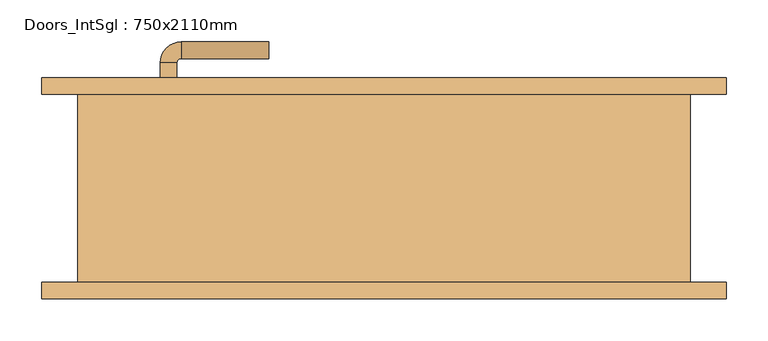
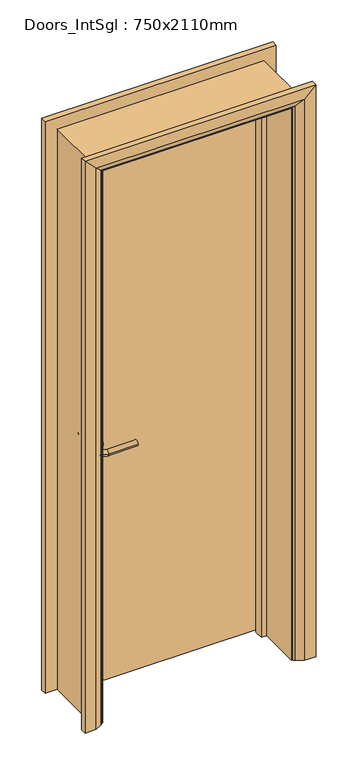
"""IFC4 building model written with IfcOpenShell, lengths in millimetres: door geometry, Doors_IntSgl : 750x2110mm."""

from ifc_helpers import new_model, si_unit, point, frame, frame_2d, origin, place, context, project, spatial, polyline, circle_curve, ellipse_curve, trimmed, segment, composite_curve, outline, extrude, faceted_brep, source, transform, mapped, element, save
from ifc_brep_helpers import plane_surface, cylinder_surface, revolved_surface, advanced_brep


def doors_intsgl_750x2110mm_542c0a28(model_context):
    return source(origin(), model_context, "Body", "SolidModel", [
        advanced_brep(
        [(-268.0, 66.5, 900.0), (-248.0, 66.5, 900.0), (-248.0, 36.5, 900.0), (-268.0, 36.5, 900.0), (-243.0, 31.5, 900.0), (-243.0, 11.5, 900.0), (-138.0, 11.5, 900.0), (-138.0, 31.5, 900.0)],
        [
            (0, 1, circle_curve(frame((-258.0, 66.5, 900.0), z_axis=(0.0, 1.0, 0.0), x_axis=(1.0, 0.0, 0.0)), 10.0)),
            (1, 0, circle_curve(frame((-258.0, 66.5, 900.0), z_axis=(0.0, 1.0, 0.0), x_axis=(1.0, 0.0, 0.0)), 10.0)),
            (1, 2),
            (2, 3, circle_curve(frame((-258.0, 36.5, 900.0), z_axis=(0.0, 1.0, 0.0), x_axis=(1.0, 0.0, 0.0)), 10.0)),
            (3, 0),
            (3, 2, circle_curve(frame((-258.0, 36.5, 900.0), z_axis=(0.0, 1.0, 0.0), x_axis=(1.0, 0.0, 0.0)), 10.0)),
            (4, 5, circle_curve(frame((-243.0, 21.5, 900.0), z_axis=(-1.0, 0.0, 0.0), x_axis=(0.0, 1.0, 0.0)), 10.0)),
            (5, 3, circle_curve(frame((-243.0, 36.5, 900.0), z_axis=(0.0, 0.0, -1.0), x_axis=(-1.0, 0.0, 0.0)), 25.0)),
            (2, 4, circle_curve(frame((-243.0, 36.5, 900.0), z_axis=(0.0, 0.0, 1.0), x_axis=(-1.0, 0.0, 0.0)), 5.0)),
            (5, 4, circle_curve(frame((-243.0, 21.5, 900.0), z_axis=(-1.0, 0.0, 0.0), x_axis=(0.0, 1.0, 0.0)), 10.0)),
            (6, 7, circle_curve(frame((-138.0, 21.5, 900.0), z_axis=(1.0, 0.0, 0.0), x_axis=(0.0, 1.0, 0.0)), 10.0)),
            (7, 6, circle_curve(frame((-138.0, 21.5, 900.0), z_axis=(1.0, 0.0, 0.0), x_axis=(0.0, 1.0, 0.0)), 10.0)),
            (4, 7),
            (6, 5),
        ],
        [
            plane_surface(frame((-258.0, 66.5, 900.0), z_axis=(0.0, 1.0, 0.0), x_axis=(0.0, 0.0, 1.0))),
            cylinder_surface(frame((-258.0, 66.5, 900.0), z_axis=(0.0, 1.0, 0.0), x_axis=(1.0, 0.0, 0.0)), 10.0),
            revolved_surface(trimmed(ellipse_curve(frame((-258.0, 36.5, 900.0), z_axis=(0.0, -1.0, 0.0), x_axis=(1.0, 0.0, 0.0)), 10.0, 10.0), [point((-268.0, 36.5, 900.0))], [point((-248.0, 36.5, 900.0))], True, "CARTESIAN"), (-243.0, 36.5, 900.0), (0.0, 0.0, -1.0)),
            revolved_surface(trimmed(ellipse_curve(frame((-258.0, 36.5, 900.0), z_axis=(0.0, -1.0, 0.0), x_axis=(1.0, 0.0, 0.0)), 10.0, 10.0), [point((-248.0, 36.5, 900.0))], [point((-268.0, 36.5, 900.0))], True, "CARTESIAN"), (-243.0, 36.5, 900.0), (0.0, 0.0, -1.0)),
            plane_surface(frame((-138.0, 21.5, 900.0), z_axis=(1.0, 0.0, 0.0), x_axis=(0.0, 0.0, 1.0))),
            cylinder_surface(frame((-243.0, 21.5, 900.0), z_axis=(-1.0, 0.0, 0.0), x_axis=(0.0, 1.0, 0.0)), 10.0),
        ],
        [
            (0, [[1, 2]]),
            (1, [[3, 4, 5, -2]]),
            (1, [[-5, 6, -3, -1]]),
            (2, [[7, 8, -4, 9]]),
            (3, [[10, -9, -6, -8]]),
            (4, [[11, 12]]),
            (5, [[13, -11, 14, -7]]),
            (5, [[-14, -12, -13, -10]]),
        ],
    ),
        extrude(outline(composite_curve([segment(trimmed(circle_curve(frame_2d((900.0, -260.5)), 30.0), [point((900.0, -290.5))], [point((900.0, -230.5))], False, "CARTESIAN"), True, "CONTINUOUS"), segment(trimmed(circle_curve(frame_2d((900.0, -260.5)), 30.0), [point((900.0, -230.5))], [point((900.0, -290.5))], False, "CARTESIAN"), True, "CONTINUOUS")], self_intersect=False)), frame((0.0, 66.5, 0.0), z_axis=(0.0, 1.0, 0.0), x_axis=(0.0, 0.0, 1.0)), (0.0, 0.0, 1.0), 8.0),
        advanced_brep(
        [(-268.0, 120.5, 900.0), (-248.0, 120.5, 900.0), (-268.0, 150.5, 900.0), (-248.0, 150.5, 900.0), (-243.0, 155.5, 900.0), (-243.0, 175.5, 900.0), (-138.0, 175.5, 900.0), (-138.0, 155.5, 900.0)],
        [
            (0, 1, circle_curve(frame((-258.0, 120.5, 900.0), z_axis=(0.0, -1.0, 0.0), x_axis=(1.0, 0.0, 0.0)), 10.0)),
            (1, 0, circle_curve(frame((-258.0, 120.5, 900.0), z_axis=(0.0, -1.0, 0.0), x_axis=(1.0, 0.0, 0.0)), 10.0)),
            (0, 2),
            (2, 3, circle_curve(frame((-258.0, 150.5, 900.0), z_axis=(0.0, -1.0, 0.0), x_axis=(1.0, 0.0, 0.0)), 10.0)),
            (3, 1),
            (3, 2, circle_curve(frame((-258.0, 150.5, 900.0), z_axis=(0.0, -1.0, 0.0), x_axis=(1.0, 0.0, 0.0)), 10.0)),
            (4, 3, circle_curve(frame((-243.0, 150.5, 900.0), z_axis=(0.0, 0.0, 1.0), x_axis=(-1.0, 0.0, 0.0)), 5.0)),
            (2, 5, circle_curve(frame((-243.0, 150.5, 900.0), z_axis=(0.0, 0.0, -1.0), x_axis=(-1.0, 0.0, 0.0)), 25.0)),
            (5, 4, circle_curve(frame((-243.0, 165.5, 900.0), z_axis=(-1.0, 0.0, 0.0), x_axis=(0.0, -1.0, 0.0)), 10.0)),
            (4, 5, circle_curve(frame((-243.0, 165.5, 900.0), z_axis=(-1.0, 0.0, 0.0), x_axis=(0.0, -1.0, 0.0)), 10.0)),
            (6, 7, circle_curve(frame((-138.0, 165.5, 900.0), z_axis=(1.0, 0.0, 0.0), x_axis=(0.0, -1.0, 0.0)), 10.0)),
            (7, 6, circle_curve(frame((-138.0, 165.5, 900.0), z_axis=(1.0, 0.0, 0.0), x_axis=(0.0, -1.0, 0.0)), 10.0)),
            (5, 6),
            (7, 4),
        ],
        [
            plane_surface(frame((-258.0, 120.5, 900.0), z_axis=(0.0, -1.0, 0.0), x_axis=(0.0, 0.0, 1.0))),
            cylinder_surface(frame((-258.0, 120.5, 900.0), z_axis=(0.0, -1.0, 0.0), x_axis=(1.0, 0.0, 0.0)), 10.0),
            revolved_surface(trimmed(ellipse_curve(frame((-258.0, 150.5, 900.0), z_axis=(0.0, -1.0, 0.0), x_axis=(1.0, 0.0, 0.0)), 10.0, 10.0), [point((-268.0, 150.5, 900.0))], [point((-248.0, 150.5, 900.0))], True, "CARTESIAN"), (-243.0, 150.5, 900.0), (0.0, 0.0, -1.0)),
            revolved_surface(trimmed(ellipse_curve(frame((-258.0, 150.5, 900.0), z_axis=(0.0, -1.0, 0.0), x_axis=(1.0, 0.0, 0.0)), 10.0, 10.0), [point((-248.0, 150.5, 900.0))], [point((-268.0, 150.5, 900.0))], True, "CARTESIAN"), (-243.0, 150.5, 900.0), (0.0, 0.0, -1.0)),
            plane_surface(frame((-138.0, 165.5, 900.0), z_axis=(1.0, 0.0, 0.0), x_axis=(0.0, 0.0, 1.0))),
            cylinder_surface(frame((-243.0, 165.5, 900.0), z_axis=(-1.0, 0.0, 0.0), x_axis=(0.0, -1.0, 0.0)), 10.0),
        ],
        [
            (0, [[1, 2]]),
            (1, [[-1, 3, 4, 5]]),
            (1, [[-2, -5, 6, -3]]),
            (2, [[7, -4, 8, 9]]),
            (3, [[-8, -6, -7, 10]]),
            (4, [[11, 12]]),
            (5, [[-9, 13, -12, 14]]),
            (5, [[-10, -14, -11, -13]]),
        ],
    ),
        extrude(outline(composite_curve([segment(trimmed(circle_curve(frame_2d((900.0, -260.5)), 30.0), [point((900.0, -290.5))], [point((900.0, -230.5))], False, "CARTESIAN"), True, "CONTINUOUS"), segment(trimmed(circle_curve(frame_2d((900.0, -260.5)), 30.0), [point((900.0, -230.5))], [point((900.0, -290.5))], False, "CARTESIAN"), True, "CONTINUOUS")], self_intersect=False)), frame((0.0, 112.5, 0.0), z_axis=(0.0, 1.0, 0.0), x_axis=(0.0, 0.0, 1.0)), (0.0, 0.0, 1.0), 8.0),
        extrude(outline(polyline([(333.0, 74.5), (-333.0, 74.5), (-333.0, 112.5), (333.0, 112.5), (333.0, 74.5)])), frame((0.0, 0.0, 8.0), z_axis=(0.0, 0.0, 1.0), x_axis=(1.0, 0.0, 0.0)), (0.0, 0.0, 1.0), 2060.0),
        advanced_brep(
        [(410.0, 132.5, 0.0), (410.0, 112.5, 0.0), (340.0, 112.5, 0.0), (344.0, 118.5, 0.0), (370.0, 132.5, 0.0), (410.0, 132.5, 2145.0), (410.0, 112.5, 2145.0), (-410.0, 112.5, 2145.0), (-410.0, 112.5, 0.0), (-340.0, 112.5, 0.0), (-340.0, 112.5, 2075.0), (340.0, 112.5, 2075.0), (344.0, 118.5, 2079.0), (370.0, 132.5, 2105.0), (-370.0, 132.5, 2105.0), (-370.0, 132.5, 0.0), (-410.0, 132.5, 0.0), (-410.0, 132.5, 2145.0), (-344.0, 118.5, 2079.0), (-344.0, 118.5, 0.0)],
        [
            (0, 1),
            (1, 2),
            (2, 3, circle_curve(frame((348.0, 111.5, 0.0), z_axis=(0.0, 0.0, -1.0), x_axis=(1.0, 0.0, 0.0)), 8.0622577)),
            (3, 4),
            (4, 0),
            (0, 5),
            (5, 6),
            (6, 1),
            (6, 7),
            (7, 8),
            (8, 9),
            (9, 10),
            (10, 11),
            (11, 2),
            (11, 12, ellipse_curve(frame((348.0, 111.5, 2083.0), z_axis=(0.7071067811865475, 0.0, -0.7071067811865475), x_axis=(-0.7071067811865474, 0.0, -0.7071067811865476)), 11.4017543, 8.0622577)),
            (12, 3),
            (12, 13),
            (13, 4),
            (13, 14),
            (14, 15),
            (15, 16),
            (16, 17),
            (17, 5),
            (17, 7),
            (10, 18, ellipse_curve(frame((-348.0, 111.5, 2083.0), z_axis=(0.7071067811865475, 0.0, 0.7071067811865475), x_axis=(0.7071067811865476, 0.0, -0.7071067811865474)), 11.4017543, 8.0622577)),
            (18, 12),
            (18, 14),
            (15, 19),
            (19, 9, circle_curve(frame((-348.0, 111.5, 0.0), z_axis=(0.0, 0.0, -1.0), x_axis=(-1.0, 0.0, 0.0)), 8.0622577)),
            (8, 16),
            (19, 18),
        ],
        [
            plane_surface(frame((340.0, 112.5, 0.0), z_axis=(0.0, 0.0, -1.0), x_axis=(0.0, -1.0, 0.0))),
            plane_surface(frame((410.0, 132.5, 0.0), z_axis=(1.0, 0.0, 0.0), x_axis=(0.0, 0.0, 1.0))),
            plane_surface(frame((410.0, 112.5, 0.0), z_axis=(0.0, -1.0, 0.0), x_axis=(0.0, 0.0, 1.0))),
            cylinder_surface(frame((348.0, 111.5, 0.0), z_axis=(0.0, 0.0, -1.0), x_axis=(1.0, 0.0, 0.0)), 8.0622577),
            plane_surface(frame((344.0, 118.5, 0.0), z_axis=(-0.4740998230350126, 0.880471099922178, 0.0), x_axis=(0.0, 0.0, 1.0))),
            plane_surface(frame((370.0, 132.5, 0.0), z_axis=(0.0, 1.0, 0.0), x_axis=(0.0, 0.0, 1.0))),
            plane_surface(frame((410.0, 132.5, 2145.0), z_axis=(0.0, 0.0, 1.0), x_axis=(-1.0, 0.0, 0.0))),
            cylinder_surface(frame((340.0, 111.5, 2083.0), z_axis=(1.0, 0.0, 0.0), x_axis=(0.0, 0.0, 1.0)), 8.0622577),
            plane_surface(frame((344.0, 118.5, 2079.0), z_axis=(0.0, 0.8804710999221764, -0.4740998230350154), x_axis=(-1.0, 0.0, 0.0))),
            plane_surface(frame((-340.0, 112.5, 0.0), z_axis=(0.0, 0.0, -1.0), x_axis=(0.0, -1.0, 0.0))),
            plane_surface(frame((-410.0, 132.5, 2145.0), z_axis=(-1.0, 0.0, 0.0), x_axis=(0.0, 0.0, -1.0))),
            cylinder_surface(frame((-348.0, 111.5, 2075.0), z_axis=(0.0, 0.0, 1.0), x_axis=(-1.0, 0.0, 0.0)), 8.0622577),
            plane_surface(frame((-344.0, 118.5, 2079.0), z_axis=(0.47409982303501824, 0.8804710999221749, 0.0), x_axis=(0.0, 0.0, -1.0))),
        ],
        [
            (0, [[1, 2, 3, 4, 5]]),
            (1, [[-1, 6, 7, 8]]),
            (2, [[-2, -8, 9, 10, 11, 12, 13, 14]]),
            (3, [[-3, -14, 15, 16]]),
            (4, [[-4, -16, 17, 18]]),
            (5, [[-5, -18, 19, 20, 21, 22, 23, -6]]),
            (6, [[-7, -23, 24, -9]]),
            (7, [[-15, -13, 25, 26]]),
            (8, [[-17, -26, 27, -19]]),
            (9, [[-21, 28, 29, -11, 30]]),
            (10, [[-24, -22, -30, -10]]),
            (11, [[-25, -12, -29, 31]]),
            (12, [[-27, -31, -28, -20]]),
        ],
    ),
        extrude(outline(polyline([(0.0, -335.0), (0.0, -316.0), (2051.0, -316.0), (2051.0, 316.0), (0.0, 316.0), (0.0, 335.0), (2070.0, 335.0), (2070.0, -335.0), (0.0, -335.0)])), frame((0.0, 40.5, 0.0), z_axis=(0.0, 1.0, 0.0), x_axis=(0.0, 0.0, 1.0)), (0.0, 0.0, 1.0), 32.0),
        advanced_brep(
        [(-410.0, -132.5, 0.0), (-410.0, -112.5, 0.0), (-340.0, -112.5, 0.0), (-344.0, -118.5, 0.0), (-370.0, -132.5, 0.0), (-410.0, -132.5, 2145.0), (-410.0, -112.5, 2145.0), (-340.0, -112.5, 2075.0), (-344.0, -118.5, 2079.0), (-370.0, -132.5, 2105.0), (410.0, -132.5, 2145.0), (410.0, -112.5, 2145.0), (340.0, -112.5, 2075.0), (344.0, -118.5, 2079.0), (370.0, -132.5, 2105.0), (410.0, -132.5, 0.0), (370.0, -132.5, 0.0), (344.0, -118.5, 0.0), (340.0, -112.5, 0.0), (410.0, -112.5, 0.0)],
        [
            (0, 1),
            (1, 2),
            (2, 3, circle_curve(frame((-348.0, -111.5, 0.0), z_axis=(0.0, 0.0, -1.0), x_axis=(-1.0, 0.0, 0.0)), 8.0622577)),
            (3, 4),
            (4, 0),
            (0, 5),
            (5, 6),
            (6, 1),
            (6, 7),
            (7, 2),
            (7, 8, ellipse_curve(frame((-348.0, -111.5, 2083.0), z_axis=(-0.7071067811865475, 0.0, -0.7071067811865475), x_axis=(0.7071067811865474, 0.0, -0.7071067811865476)), 11.4017543, 8.0622577)),
            (8, 3),
            (8, 9),
            (9, 4),
            (9, 5),
            (5, 10),
            (10, 11),
            (11, 6),
            (11, 12),
            (12, 7),
            (12, 13, ellipse_curve(frame((348.0, -111.5, 2083.0), z_axis=(-0.7071067811865475, 0.0, 0.7071067811865475), x_axis=(-0.7071067811865476, 0.0, -0.7071067811865474)), 11.4017543, 8.0622577)),
            (13, 8),
            (13, 14),
            (14, 9),
            (14, 10),
            (15, 16),
            (16, 17),
            (17, 18, circle_curve(frame((348.0, -111.5, 0.0), z_axis=(0.0, 0.0, -1.0), x_axis=(1.0, 0.0, 0.0)), 8.0622577)),
            (18, 19),
            (19, 15),
            (10, 15),
            (19, 11),
            (18, 12),
            (17, 13),
            (16, 14),
        ],
        [
            plane_surface(frame((-340.0, -185.3010989, 0.0), z_axis=(0.0, 0.0, -1.0), x_axis=(1.0, 0.0, 0.0))),
            plane_surface(frame((-410.0, -132.5, 0.0), z_axis=(-1.0, 0.0, 0.0), x_axis=(0.0, 0.0, 1.0))),
            plane_surface(frame((-410.0, -112.5, 0.0), z_axis=(0.0, 1.0, 0.0), x_axis=(0.0, 0.0, 1.0))),
            cylinder_surface(frame((-348.0, -111.5, 0.0), z_axis=(0.0, 0.0, -1.0), x_axis=(-1.0, 0.0, 0.0)), 8.0622577),
            plane_surface(frame((-344.0, -118.5, 0.0), z_axis=(0.4740998230350183, -0.8804710999221749, 0.0), x_axis=(0.0, 0.0, 1.0))),
            plane_surface(frame((-370.0, -132.5, 0.0), z_axis=(0.0, -1.0, 0.0), x_axis=(0.0, 0.0, 1.0))),
            plane_surface(frame((-410.0, -132.5, 2145.0), z_axis=(0.0, 0.0, 1.0), x_axis=(1.0, 0.0, 0.0))),
            plane_surface(frame((-410.0, -112.5, 2145.0), z_axis=(0.0, 1.0, 0.0), x_axis=(1.0, 0.0, 0.0))),
            cylinder_surface(frame((-340.0, -111.5, 2083.0), z_axis=(-1.0, 0.0, 0.0), x_axis=(0.0, 0.0, 1.0)), 8.0622577),
            plane_surface(frame((-344.0, -118.5, 2079.0), z_axis=(0.0, -0.8804710999221749, -0.4740998230350183), x_axis=(1.0, 0.0, 0.0))),
            plane_surface(frame((-370.0, -132.5, 2105.0), z_axis=(0.0, -1.0, 0.0), x_axis=(1.0, 0.0, 0.0))),
            plane_surface(frame((340.0, -185.3010989, 0.0), z_axis=(0.0, 0.0, -1.0), x_axis=(-1.0, 0.0, 0.0))),
            plane_surface(frame((410.0, -132.5, 2145.0), z_axis=(1.0, 0.0, 0.0), x_axis=(0.0, 0.0, -1.0))),
            plane_surface(frame((410.0, -112.5, 2145.0), z_axis=(0.0, 1.0, 0.0), x_axis=(0.0, 0.0, -1.0))),
            cylinder_surface(frame((348.0, -111.5, 2075.0), z_axis=(0.0, 0.0, 1.0), x_axis=(1.0, 0.0, 0.0)), 8.0622577),
            plane_surface(frame((344.0, -118.5, 2079.0), z_axis=(-0.4740998230350183, -0.8804710999221749, 0.0), x_axis=(0.0, 0.0, -1.0))),
            plane_surface(frame((370.0, -132.5, 2105.0), z_axis=(0.0, -1.0, 0.0), x_axis=(0.0, 0.0, -1.0))),
        ],
        [
            (0, [[1, 2, 3, 4, 5]]),
            (1, [[-1, 6, 7, 8]]),
            (2, [[-2, -8, 9, 10]]),
            (3, [[-3, -10, 11, 12]]),
            (4, [[-4, -12, 13, 14]]),
            (5, [[-5, -14, 15, -6]]),
            (6, [[-7, 16, 17, 18]]),
            (7, [[-9, -18, 19, 20]]),
            (8, [[-11, -20, 21, 22]]),
            (9, [[-13, -22, 23, 24]]),
            (10, [[-15, -24, 25, -16]]),
            (11, [[26, 27, 28, 29, 30]]),
            (12, [[-17, 31, -30, 32]]),
            (13, [[-19, -32, -29, 33]]),
            (14, [[-21, -33, -28, 34]]),
            (15, [[-23, -34, -27, 35]]),
            (16, [[-25, -35, -26, -31]]),
        ],
    ),
        faceted_brep([(-335.0, 112.5, 0.0), (-335.0, -112.5, 0.0), (-367.0, -112.5, 0.0), (-367.0, 112.5, 0.0), (-335.0, 112.5, 2070.0), (-335.0, -112.5, 2070.0), (-367.0, -112.5, 2102.0), (-367.0, 112.5, 2102.0), (335.0, 112.5, 2070.0), (335.0, -112.5, 2070.0), (367.0, -112.5, 2102.0), (367.0, 112.5, 2102.0), (335.0, 112.5, 0.0), (367.0, 112.5, 0.0), (367.0, -112.5, 0.0), (335.0, -112.5, 0.0)], [[[0, 1, 2, 3]], [[1, 0, 4, 5]], [[2, 1, 5, 6]], [[3, 2, 6, 7]], [[0, 3, 7, 4]], [[5, 4, 8, 9]], [[6, 5, 9, 10]], [[7, 6, 10, 11]], [[4, 7, 11, 8]], [[12, 13, 14, 15]], [[9, 8, 12, 15]], [[10, 9, 15, 14]], [[11, 10, 14, 13]], [[8, 11, 13, 12]]]),
    ])


if __name__ == "__main__":
    model = new_model("IFC4")
    model_context = context("Model", 3, world=origin())
    ifc_project = project(units=[si_unit("LENGTHUNIT", "METRE", prefix="MILLI")], contexts=[model_context])
    site = spatial("IfcSite", under=ifc_project)
    building = spatial("IfcBuilding", under=site)
    placement = place(None, origin())
    doors_intsgl_750x2110mm_shape = doors_intsgl_750x2110mm_542c0a28(model_context)
    element("IfcDoor", 1, ObjectType="Doors_IntSgl : 750x2110mm", at=placement, inside=building, context=model_context, shape_type="MappedRepresentation", body=[
        mapped(doors_intsgl_750x2110mm_shape, transform((0.0, 0.0, 0.0), x_axis=(1.0, 0.0, 0.0), y_axis=(0.0, 1.0, 0.0), z_axis=(0.0, 0.0, 1.0))),
    ])
    save(model, "model.ifc")

# Revit data of these elements
# Type "Doors_IntSgl : 750x2110mm"
#   Construction Type Id = "MDOOR"
#   Type Mark = "42"
#   Type Comments = "Internal Single"
#   Operation = "SingleSwingRight"
#   Manufacturer = "Revit"
#   Keynote = "L20"
#   Description = "Internal Single Door"
#   Analytic Construction = "Metal"
#   UnderCut = 8 mm
#   Tolerance = 2 mm
#   Thickness = 38 mm
#   Thermal Resistance (R) = 0.270117 (m²·K)/W
#   Structural Tolerance = 8 mm
#   StopDepth = 32 mm
#   Stop Thickness = 19 mm
#   Rough Width = 750 mm
#   Rough Height = 2110 mm
#   Height to Top Lock Rail = 1000 mm
#   Heat Transfer Coefficient (U) = 3.7021 W/(m²·K)
#   Handle Z Distance = 900 mm
#   Handle X Distance = 75 mm
#   Frame Thickness = 32 mm
#   Door Panel Width = 666 mm
#   Door Panel Thickness = 38 mm
#   Door Panel Offset = 0 mm
#   Height = 2110 mm
#   Width = 750 mm
#   Door Panel Height = 2060 mm
#   Architrave Setback = 5 mm
#   Define Thermal Properties by = 1
#   Vis - Ironmongery = yes
#   Material Ironmongery = Door - Handle
#   Material Frame = Door - Frame/Mullion (1)
#   Material Door = Door - Panel
#   Material Architrave = Door - Architrave
#   Visual Light Transmittance = 0
#   Solar Heat Gain Coefficient = 0
#   Function = (empty or 0)
#   Wall Closure = (empty or 0)
# Element 1 (IfcDoor, "Doors_IntSgl : 750x2110mm")
#   Materials on its faces: "Door - Architrave", "Door - Handle", "Door - Frame/Mullion (1)", "Door - Panel"
# Materials
#   "Door - Handle": colour RGB 0 0 0, transparency 0, Keynote = "P21", Cost = 0
#   "Door - Frame/Mullion (1)": class "Wood", colour RGB 212 179 113, transparency 0, Keynote = "L20", Cost = 0
#   "Door - Panel": class "Wood", colour RGB 210 159 95, transparency 0, Keynote = "L20", Cost = 0
#   "Door - Architrave": class "Wood", colour RGB 154 90 5, transparency 0, Keynote = "P20", Cost = 0
